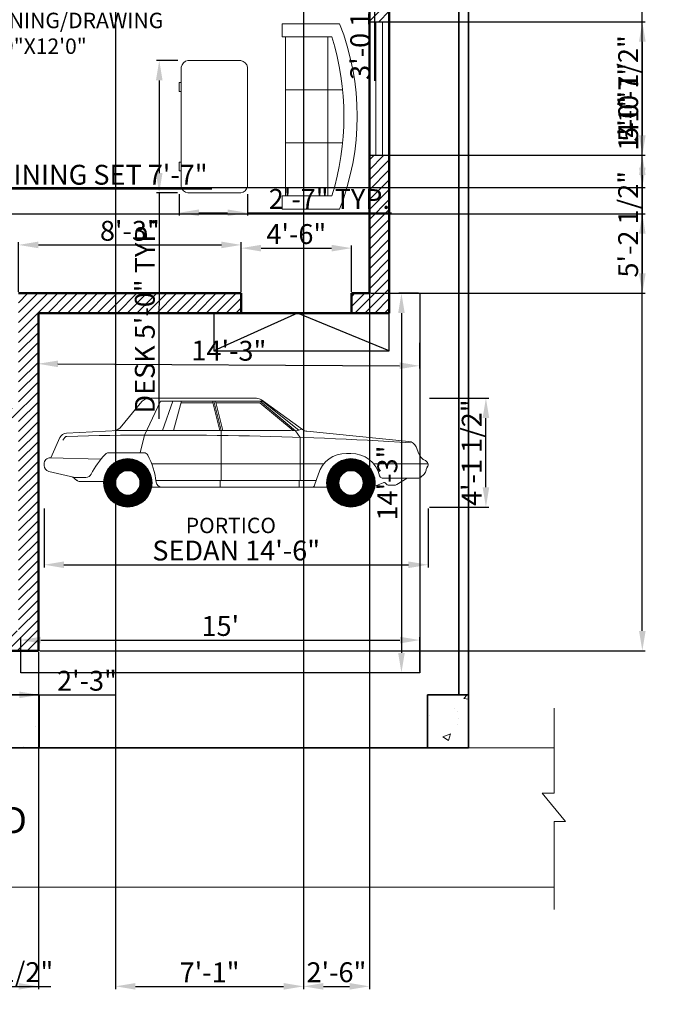
# Model space of a CAD drawing. Units: inches. Extents: x 53662 to 54269, y 37303 to 38048.
# Tile 4 of 6: x 53979 to 54269, y 37303 to 37749. Entities that reach past the tile are written whole.
import ezdxf

# ---------------------------------------------------------------- set-up
doc = ezdxf.new("R2010")
doc.units = ezdxf.units.IN
for name, color, linetype, lineweight in [('A-ANNO-DIMS', 2, 'Continuous', 18), ('A-ANNO-TEXT', 7, 'Continuous', 25), ('A-AREA-IDEN', 7, 'Continuous', 25), ('A-EQPM-VEHI', 8, 'Continuous', 13), ('A-FLOR', 7, 'Continuous', 25), ('A-FLOR-STRS', 7, 'Continuous', 25), ('A-FURN', 8, 'Continuous', 18), ('A-GLAZ', 4, 'Continuous', 18), ('A-WALL', 7, 'Continuous', 50), ('C-PROP', 7, 'Continuous', 35), ('C-ROAD', 8, 'Continuous', 18), ('C-SITE-PATT', 8, 'Continuous', 13)]:
    doc.layers.add(name, color=color, linetype=linetype, lineweight=lineweight)
doc.layers.add('A-WALL-PATT', color=244, linetype='Continuous', lineweight=13, true_color=0x991b1e)
doc.styles.get("Standard").update_dxf_attribs({"font": 'arial.ttf'})
doc.dimstyles.new('ISO-25', dxfattribs={"dimtxt": 9, "dimasz": 9, "dimexe": 1.25, "dimexo": 0.625, "dimtad": 1, "dimdec": 1, "dimrnd": 9, "dimlunit": 3, "dimtxsty": 'Standard', "dimcen": 2.5, "dimadec": 0, "dimazin": 0, "dimtfac": 1, "dimtdec": 1, "dimtmove": 0, "dimatfit": 3, "dimfxl": 1, "dimarcsym": 0})

# ---------------------------------------------------------------- blocks, each defined once
blk = doc.blocks.new('Car - sedan  side')
for p, q in [((-77.81, 49.34), (-126.58, 49.34)), ((-139.53, 35.99), (-129.64, 47.91)), ((-128.57, 32.64), (-121.22, 48.02)), ((-74.7, 48.02), (-121.22, 48.02)), ((-120.32, 34.67), (-115.67, 48.02)), ((-115.4, 34.67), (-111.74, 48.02)), ((-97.55, 47.3), (-111.94, 47.3)), ((-94.41, 34.67), (-97.73, 48.02)), ((-93.72, 34.67), (-97.04, 48.02)), ((-93.03, 34.67), (-96.34, 48.02)), ((-76.26, 47.3), (-96.16, 47.3)), ((-61.08, 34.66), (-76.26, 47.3)), ((-60.02, 34.65), (-76.07, 48.02)), ((-56.87, 35.13), (-75.48, 48.59)), ((-58.54, 34.93), (-74.99, 48.02)), ((-170.93, 22.32), (-166.81, 31.56)), ((-164.57, 31.6), (-165.48, 30.35)), ((-140.23, 34.67), (-163.88, 33.56)), ((-62.28, 34.67), (-140.23, 34.67)), ((-130.39, 24.63), (-128.57, 32.64)), ((-93.72, 19.62), (-93.72, 34.67)), ((-62.28, 34.67), (-60.02, 34.65)), ((-60.02, 34.65), (-58.54, 34.93)), ((-57.97, 31.61), (-60.02, 34.65)), ((-57.21, 35.38), (-58.54, 34.93)), ((-57.97, 19.62), (-57.97, 31.61)), ((-54.93, 34.4), (-8.75, 29.8)), ((-4.21, 24.18), (-5.42, 27.27)), ((-148.26, 21.7), (-171.11, 22.33)), ((-128.78, 24.63), (-144.79, 24.63)), ((-36.97, 24.38), (-34.94, 24.38)), ((-174, 19.51), (-174, 18.91)), ((-47.2, 19.62), (-125.23, 19.62)), ((-93.72, 12.14), (-93.72, 19.62)), ((-57.97, 12.14), (-57.97, 19.62)), ((0, 19.62), (-24.7, 19.62)), ((-160.12, 13.48), (-171.81, 16.16)), ((-159.22, 12.14), (-161.08, 13.7)), ((-155.01, 13.48), (-160.12, 13.48)), ((-51.4, 9.89), (-49.69, 15.14)), ((-3.22, 13.59), (-1.77, 14.97)), ((-147.03, 11.6), (-157.73, 11.6)), ((-120.62, 9.03), (-125.23, 9.03)), ((-50.67, 12.14), (-123.32, 12.14)), ((-45.76, 9.03), (-120.62, 9.03)), ((-94.21, 9.03), (-94.21, 12.14)), ((-58.39, 9.03), (-58.39, 12.14)), ((-20.36, 11.06), (-24.06, 9.44)), ((-4.23, 13.19), (-20.72, 13.19)), ((-18.83, 10.42), (-19.11, 10.76)), ((-14.68, 10.03), (-18.01, 10.03)), ((-9.5, 13.19), (-14.1, 10.2))]:
    blk.add_line(p, q)
at = {"const_width": 5.49}
for points in [[(-127.8, 11, -1), (-144.3, 11, -1)], [(-26.69, 11, -1), (-43.19, 11, -1)]]:
    blk.add_lwpolyline(points, format="xyb", close=True, dxfattribs=at)
for centre, radius in [((-136.05, 11), 11), ((-34.94, 11), 11), ((-136.05, 11), 5.51), ((-34.94, 11), 5.51)]:
    blk.add_circle(centre, radius)
for centre, radius, start, end in [((-126.58, 45.38), 3.97, 90, 140.3029), ((-77.81, 45.38), 3.97, 54.135, 90), ((-142.58, 38.53), 3.97, 272.6827, 320.3029), ((-163.72, 30.18), 3.38, 92.6827, 155.9736), ((-163.62, 30.91), 1.17, 91.491, 143.9553), ((-118.51, -1702.12), 1734.79, 86.34698, 91.49105), ((-54.54, 38.35), 3.97, 234.135, 264.3123), ((-9.15, 25.82), 4, 21.3107, 84.3123), ((-171.18, 19.51), 2.82, 88.4193, 180), ((-118.09, -2.78), 38.85, 136.3964, 152.9097), ((-144.79, 22.64), 1.98, 90, 136.3964), ((-128.78, 22.64), 1.98, 28.1371, 90), ((-157.14, 7.48), 34.14, 6.5135, 28.1371), ((-36.97, 11), 13.38, 90, 161.9732), ((-34.94, 11), 13.38, 13.5864, 90), ((0.9, 26.18), 5.49, 201.3107, 247.7048), ((-171.18, 18.91), 2.82, 180, 257.0905), ((-1.92, 19.3), 1.94, 325.3744, 67.7048), ((2.46, 16.28), 3.37, 145.3744, 172.3839), ((-155.01, 16.1), 2.62, 270, 332.9097), ((-20.72, 14.43), 1.24, 193.5864, 270), ((-4.23, 14.65), 1.46, 270, 313.7173), ((-3.82, 17.12), 2.96, 313.7173, 352.3839), ((-157.73, 13.93), 2.32, 230.1291, 270), ((-120.62, 11.65), 2.62, 186.5135, 270), ((-52.58, 10.27), 1.24, 270, 341.9732), ((-19.93, 10.09), 1.06, 39.301, 113.7159), ((-18.01, 11.09), 1.06, 219.301, 270), ((-14.68, 11.09), 1.06, 270, 303.047)]:
    blk.add_arc(centre, radius, start, end)
blk = doc.blocks.new('Sofa - Roundback 7 ft.')
for p, q in [((-12.00002, -32.4421), (-12.00003, -6.5971)), ((11.99997, -32.4421), (11.99998, -6.5971)), ((-36.000027, -34), (-36.000027, -11.4696)), ((-35.999844, -13.3819), (35.9998, -13.3819)), ((35.99998, -34), (35.99998, -11.4696)), ((-36.000027, -32.4421), (35.99998, -32.4421))]:
    blk.add_line(p, q)
for points in [[(-36.000027, -34), (-42.000027, -34), (-42.000027, -8)], [(41.99998, -8), (41.99998, -34), (35.99998, -34)]]:
    blk.add_lwpolyline(points)
for centre, radius, start, end in [((0, -114.25), 114.25, 68.43141, 111.5686), ((-0.00001, -127.1968), 121.1968, 72.72033, 107.2797)]:
    blk.add_arc(centre, radius, start, end)
blk = doc.blocks.new('Desk - 30 x 60 in.')
for p, q in [((-26.999995, 0), (26.999995, 0)), ((-29.999995, -27), (-29.999995, -3)), ((29.999995, -3), (29.999995, -27)), ((26.999995, -30), (-26.999995, -30)), ((-20.000005, -30), (-20.000005, -31)), ((-20.000005, -31), (-16.000005, -31)), ((-16.000005, -31), (-16.000005, -30)), ((15.999995, -31), (15.999995, -30)), ((19.999995, -31), (15.999995, -31)), ((19.999995, -30), (19.999995, -31))]:
    blk.add_line(p, q)
for centre, start, end in [((-26.499995, -3.5), 98.1301, 171.8699), ((26.499995, -3.5), 8.130102, 81.8699), ((-26.499995, -26.5), 188.1301, 261.8699), ((26.499995, -26.5), 278.1301, 351.8699)]:
    blk.add_arc(centre, 3.535534, start, end)
blk = doc.blocks.new('*D19')
at = {"layer": 'A-ANNO-DIMS', "color": 0, "lineweight": -2, "transparency": 16777216}
for p, q in [((53964.39, 37443.48), (53964.39, 37444.1)), ((53973.39, 37442.85), (53978.47, 37442.85)), ((53987.47, 37442.85), (54021.8, 37442.85)), ((53987.47, 37442.23), (53987.47, 37441.6))]:
    blk.add_line(p, q, dxfattribs=at)
at = {"layer": 'A-ANNO-DIMS', "color": 0, "transparency": 16777216}
for points in [[(53973.39, 37444.35), (53973.39, 37441.35), (53964.39, 37442.85)], [(53978.47, 37444.35), (53978.47, 37441.35), (53987.47, 37442.85)]]:
    blk.add_solid(points, dxfattribs=at)
at = {"layer": 'Defpoints', "color": 0, "transparency": 16777216}
for p in [(53964.39, 37442.85), (53987.47, 37442.85), (53987.47, 37442.85)]:
    blk.add_point(p, dxfattribs=at)
at = {"layer": 'A-ANNO-DIMS', "color": 0, "transparency": 16777216, "insert": (54009.13, 37448.08), "char_height": 9, "attachment_point": 5}
blk.add_mtext('2\'-3"', dxfattribs=at)
blk = doc.blocks.new('*D20')
at = {"layer": 'A-ANNO-DIMS', "color": 0, "lineweight": -2, "transparency": 16777216}
for p, q in [((53979.17, 37453.49), (53979.17, 37468.93)), ((53988.17, 37467.68), (54150.95, 37467.68)), ((54159.95, 37453.49), (54159.95, 37468.93))]:
    blk.add_line(p, q, dxfattribs=at)
at = {"layer": 'A-ANNO-DIMS', "color": 0, "transparency": 16777216}
for points in [[(53988.17, 37469.18), (53988.17, 37466.18), (53979.17, 37467.68)], [(54150.95, 37469.18), (54150.95, 37466.18), (54159.95, 37467.68)]]:
    blk.add_solid(points, dxfattribs=at)
at = {"layer": 'Defpoints', "color": 0, "transparency": 16777216}
for p in [(54159.95, 37467.68), (53979.17, 37452.86), (54159.95, 37452.86)]:
    blk.add_point(p, dxfattribs=at)
at = {"layer": 'A-ANNO-DIMS', "color": 0, "transparency": 16777216, "insert": (54069.56, 37472.9), "char_height": 9, "attachment_point": 5}
blk.add_mtext("15'", dxfattribs=at)
blk = doc.blocks.new('*D21')
at = {"layer": 'A-ANNO-DIMS', "color": 0, "lineweight": -2, "transparency": 16777216}
for p, q in [((54159.33, 37624.86), (54150.4, 37624.86)), ((54151.65, 37615.86), (54151.65, 37461.86)), ((54159.33, 37452.86), (54150.4, 37452.86))]:
    blk.add_line(p, q, dxfattribs=at)
at = {"layer": 'A-ANNO-DIMS', "color": 0, "transparency": 16777216}
for points in [[(54150.15, 37615.86), (54153.15, 37615.86), (54151.65, 37624.86)], [(54150.15, 37461.86), (54153.15, 37461.86), (54151.65, 37452.86)]]:
    blk.add_solid(points, dxfattribs=at)
at = {"layer": 'Defpoints', "color": 0, "transparency": 16777216}
for p in [(54159.95, 37624.86), (54151.65, 37452.86), (54159.95, 37452.86)]:
    blk.add_point(p, dxfattribs=at)
at = {"layer": 'A-ANNO-DIMS', "color": 0, "transparency": 16777216, "insert": (54146.43, 37538.86), "char_height": 9, "attachment_point": 5, "rotation": 90}
blk.add_mtext('14\'-3"', dxfattribs=at)
blk = doc.blocks.new('*D23')
at = {"layer": 'A-ANNO-DIMS', "color": 0, "lineweight": -2, "transparency": 16777216}
for p, q in [((53978.11, 37625.49), (53978.11, 37648.03)), ((53987.11, 37646.78), (54070.03, 37646.78)), ((54079.03, 37625.49), (54079.03, 37648.03))]:
    blk.add_line(p, q, dxfattribs=at)
at = {"layer": 'A-ANNO-DIMS', "color": 0, "transparency": 16777216}
for points in [[(53987.11, 37648.28), (53987.11, 37645.28), (53978.11, 37646.78)], [(54070.03, 37648.28), (54070.03, 37645.28), (54079.03, 37646.78)]]:
    blk.add_solid(points, dxfattribs=at)
at = {"layer": 'Defpoints', "color": 0, "transparency": 16777216}
for p in [(54079.03, 37646.78), (53978.11, 37624.86), (54079.03, 37624.86)]:
    blk.add_point(p, dxfattribs=at)
at = {"layer": 'A-ANNO-DIMS', "color": 0, "transparency": 16777216, "insert": (54028.57, 37652), "char_height": 9, "attachment_point": 5}
blk.add_mtext('8\'-3"', dxfattribs=at)
blk = doc.blocks.new('*D24')
at = {"layer": 'A-ANNO-DIMS', "color": 0, "lineweight": -2, "transparency": 16777216}
for p, q in [((54079.03, 37625.49), (54079.03, 37646.56)), ((54128.99, 37625.49), (54128.99, 37646.56)), ((54088.03, 37645.31), (54119.99, 37645.31))]:
    blk.add_line(p, q, dxfattribs=at)
at = {"layer": 'A-ANNO-DIMS', "color": 0, "transparency": 16777216}
for points in [[(54088.03, 37646.81), (54088.03, 37643.81), (54079.03, 37645.31)], [(54119.99, 37646.81), (54119.99, 37643.81), (54128.99, 37645.31)]]:
    blk.add_solid(points, dxfattribs=at)
at = {"layer": 'Defpoints', "color": 0, "transparency": 16777216}
for p in [(54128.99, 37645.31), (54079.03, 37624.86), (54128.99, 37624.86)]:
    blk.add_point(p, dxfattribs=at)
at = {"layer": 'A-ANNO-DIMS', "color": 0, "transparency": 16777216, "insert": (54104.01, 37650.53), "char_height": 9, "attachment_point": 5}
blk.add_mtext('4\'-6"', dxfattribs=at)
blk = doc.blocks.new('*D25')
at = {"layer": 'A-ANNO-DIMS', "color": 0, "lineweight": -2, "transparency": 16777216}
for p, q in [((53987.11, 37615.24), (53986.99, 37591.66)), ((54159.95, 37614.31), (54159.82, 37590.73)), ((53995.99, 37592.86), (54150.83, 37592.03))]:
    blk.add_line(p, q, dxfattribs=at)
at = {"layer": 'A-ANNO-DIMS', "color": 0, "transparency": 16777216}
for points in [[(53996, 37594.36), (53995.98, 37591.36), (53986.99, 37592.91)], [(54150.84, 37593.53), (54150.82, 37590.53), (54159.83, 37591.98)]]:
    blk.add_solid(points, dxfattribs=at)
at = {"layer": 'Defpoints', "color": 0, "transparency": 16777216}
for p in [(53987.11, 37615.86), (54159.95, 37614.93), (54159.83, 37591.98)]:
    blk.add_point(p, dxfattribs=at)
at = {"layer": 'A-ANNO-DIMS', "color": 0, "transparency": 16777216, "insert": (54073.44, 37597.67), "char_height": 9, "attachment_point": 5, "rotation": 359.6927}
blk.add_mtext('14\'-3"', dxfattribs=at)
blk = doc.blocks.new('*D31')
at = {"layer": 'A-ANNO-DIMS', "color": 0, "lineweight": -2, "transparency": 16777216}
for p, q in [((54127.43, 37843.84), (54140.66, 37843.84)), ((54139.41, 37834.84), (54139.41, 37816.17)), ((54127.43, 37807.17), (54140.66, 37807.17)), ((54139.41, 37807.17), (54139.41, 37721.1))]:
    blk.add_line(p, q, dxfattribs=at)
at = {"layer": 'A-ANNO-DIMS', "color": 0, "transparency": 16777216}
for points in [[(54137.91, 37834.84), (54140.91, 37834.84), (54139.41, 37843.84)], [(54137.91, 37816.17), (54140.91, 37816.17), (54139.41, 37807.17)]]:
    blk.add_solid(points, dxfattribs=at)
at = {"layer": 'Defpoints', "color": 0, "transparency": 16777216}
for p in [(54126.81, 37843.84), (54126.81, 37807.17), (54139.41, 37807.17)]:
    blk.add_point(p, dxfattribs=at)
at = {"layer": 'A-ANNO-DIMS', "color": 0, "transparency": 16777216, "insert": (54134.13, 37759.63), "char_height": 9, "attachment_point": 5, "rotation": 90}
blk.add_mtext('3\'-0 1/2" TYP.', dxfattribs=at)
blk = doc.blocks.new('*D32')
at = {"layer": 'A-ANNO-DIMS', "color": 0, "lineweight": -2, "transparency": 16777216}
for p, q in [((54050.27, 37730.35), (54040.65, 37730.36)), ((54041.89, 37721.36), (54041.86, 37679.36)), ((54050.23, 37670.35), (54040.6, 37670.36)), ((54041.85, 37670.36), (54041.77, 37567.96))]:
    blk.add_line(p, q, dxfattribs=at)
at = {"layer": 'A-ANNO-DIMS', "color": 0, "transparency": 16777216}
for points in [[(54040.39, 37721.36), (54043.39, 37721.35), (54041.9, 37730.36)], [(54040.36, 37679.36), (54043.36, 37679.35), (54041.85, 37670.36)]]:
    blk.add_solid(points, dxfattribs=at)
at = {"layer": 'Defpoints', "color": 0, "transparency": 16777216}
for p in [(54050.9, 37730.35), (54041.85, 37670.36), (54050.85, 37670.35)]:
    blk.add_point(p, dxfattribs=at)
at = {"layer": 'A-ANNO-DIMS', "color": 0, "transparency": 16777216, "insert": (54036.53, 37614.66), "char_height": 9, "attachment_point": 5, "rotation": 89.9534}
blk.add_mtext('DESK 5\'-0" TYP.', dxfattribs=at)
blk = doc.blocks.new('*D33')
at = {"layer": 'A-ANNO-DIMS', "color": 0, "lineweight": -2, "transparency": 16777216}
for p, q in [((54050.85, 37669.72), (54050.84, 37660.1)), ((54081.85, 37669.7), (54081.84, 37660.07)), ((54059.84, 37661.34), (54072.84, 37661.33)), ((54081.84, 37661.32), (54147.11, 37661.27))]:
    blk.add_line(p, q, dxfattribs=at)
at = {"layer": 'A-ANNO-DIMS', "color": 0, "transparency": 16777216}
for points in [[(54059.84, 37662.84), (54059.84, 37659.84), (54050.84, 37661.35)], [(54072.84, 37662.83), (54072.84, 37659.83), (54081.84, 37661.32)]]:
    blk.add_solid(points, dxfattribs=at)
at = {"layer": 'Defpoints', "color": 0, "transparency": 16777216}
for p in [(54050.85, 37670.35), (54081.85, 37670.32), (54081.84, 37661.32)]:
    blk.add_point(p, dxfattribs=at)
at = {"layer": 'A-ANNO-DIMS', "color": 0, "transparency": 16777216, "insert": (54118.98, 37666.44), "char_height": 9, "attachment_point": 5, "rotation": 359.9534}
blk.add_mtext('2\'-7" TYP.', dxfattribs=at)
blk = doc.blocks.new('*D34')
at = {"layer": 'A-ANNO-DIMS', "color": 0, "lineweight": -2, "transparency": 16777216}
for p, q in [((53865.53, 37685.16), (53865.53, 37670.88)), ((53956.53, 37685.16), (53956.53, 37670.88)), ((53874.53, 37672.13), (53947.53, 37672.13)), ((53956.53, 37672.13), (54065.7, 37672.13))]:
    blk.add_line(p, q, dxfattribs=at)
at = {"layer": 'A-ANNO-DIMS', "color": 0, "transparency": 16777216}
for points in [[(53874.53, 37673.63), (53874.53, 37670.63), (53865.53, 37672.13)], [(53947.53, 37673.63), (53947.53, 37670.63), (53956.53, 37672.13)]]:
    blk.add_solid(points, dxfattribs=at)
at = {"layer": 'Defpoints', "color": 0, "transparency": 16777216}
for p in [(53865.53, 37685.78), (53956.53, 37685.78), (53956.53, 37672.13)]:
    blk.add_point(p, dxfattribs=at)
at = {"layer": 'A-ANNO-DIMS', "color": 0, "transparency": 16777216, "insert": (54015.61, 37677.41), "char_height": 9, "attachment_point": 5}
blk.add_mtext('DINING SET 7\'-7"', dxfattribs=at)
blk = doc.blocks.new('*D48')
at = {"layer": 'A-ANNO-DIMS', "color": 0, "lineweight": -2, "transparency": 16777216}
for p, q in [((53989.7, 37527.31), (53989.7, 37500.56)), ((54163.81, 37527.31), (54163.81, 37500.56)), ((53998.7, 37501.81), (54154.81, 37501.81))]:
    blk.add_line(p, q, dxfattribs=at)
at = {"layer": 'A-ANNO-DIMS', "color": 0, "transparency": 16777216}
for points in [[(53998.7, 37503.31), (53998.7, 37500.31), (53989.7, 37501.81)], [(54154.81, 37503.31), (54154.81, 37500.31), (54163.81, 37501.81)]]:
    blk.add_solid(points, dxfattribs=at)
at = {"layer": 'Defpoints', "color": 0, "transparency": 16777216}
for p in [(53989.7, 37527.93), (54163.81, 37527.93), (54163.81, 37501.81)]:
    blk.add_point(p, dxfattribs=at)
at = {"layer": 'A-ANNO-DIMS', "color": 0, "transparency": 16777216, "insert": (54076.76, 37507.09), "char_height": 9, "attachment_point": 5}
blk.add_mtext('SEDAN 14\'-6"', dxfattribs=at)
blk = doc.blocks.new('*D49')
at = {"layer": 'A-ANNO-DIMS', "color": 0, "lineweight": -2, "transparency": 16777216}
for p, q in [((54164.44, 37577.28), (54191.18, 37577.28)), ((54189.93, 37536.93), (54189.93, 37568.28)), ((54164.44, 37527.93), (54191.18, 37527.93))]:
    blk.add_line(p, q, dxfattribs=at)
at = {"layer": 'A-ANNO-DIMS', "color": 0, "transparency": 16777216}
for points in [[(54188.43, 37568.28), (54191.43, 37568.28), (54189.93, 37577.28)], [(54188.43, 37536.93), (54191.43, 37536.93), (54189.93, 37527.93)]]:
    blk.add_solid(points, dxfattribs=at)
at = {"layer": 'Defpoints', "color": 0, "transparency": 16777216}
for p in [(54163.81, 37577.28), (54189.93, 37577.28), (54163.81, 37527.93)]:
    blk.add_point(p, dxfattribs=at)
at = {"layer": 'A-ANNO-DIMS', "color": 0, "transparency": 16777216, "insert": (54184.65, 37552.6), "char_height": 9, "attachment_point": 5, "rotation": 90}
blk.add_mtext('4\'-1 1/2"', dxfattribs=at)
blk = doc.blocks.new('*D51')
at = {"layer": 'A-ANNO-DIMS', "color": 0, "lineweight": -2, "transparency": 16777216}
for p, q in [((54146.74, 37961.86), (54262.07, 37961.86)), ((54260.82, 37471.86), (54260.82, 37952.86)), ((53987.74, 37462.86), (54262.07, 37462.86))]:
    blk.add_line(p, q, dxfattribs=at)
at = {"layer": 'A-ANNO-DIMS', "color": 0, "transparency": 16777216}
for points in [[(54259.32, 37952.86), (54262.32, 37952.86), (54260.82, 37961.86)], [(54259.32, 37471.86), (54262.32, 37471.86), (54260.82, 37462.86)]]:
    blk.add_solid(points, dxfattribs=at)
at = {"layer": 'Defpoints', "color": 0, "transparency": 16777216}
for p in [(54146.11, 37961.86), (54260.82, 37961.86), (53987.11, 37462.86)]:
    blk.add_point(p, dxfattribs=at)
at = {"layer": 'A-ANNO-DIMS', "color": 0, "transparency": 16777216, "insert": (54255.68, 37712.36), "char_height": 9, "attachment_point": 5, "rotation": 90}
blk.add_mtext('41\'-7"', dxfattribs=at)
blk = doc.blocks.new('*D53')
at = {"layer": 'A-ANNO-DIMS', "color": 0, "lineweight": -2, "transparency": 16777216}
for p, q in [((54260.82, 37681.86), (54260.82, 37715.19)), ((53828.74, 37672.86), (54262.07, 37672.86)), ((54260.82, 37660.86), (54260.82, 37672.86)), ((53828.74, 37660.86), (54262.07, 37660.86)), ((54260.82, 37651.86), (54260.82, 37642.86))]:
    blk.add_line(p, q, dxfattribs=at)
at = {"layer": 'A-ANNO-DIMS', "color": 0, "transparency": 16777216}
for points in [[(54259.32, 37681.86), (54262.32, 37681.86), (54260.82, 37672.86)], [(54259.32, 37651.86), (54262.32, 37651.86), (54260.82, 37660.86)]]:
    blk.add_solid(points, dxfattribs=at)
at = {"layer": 'Defpoints', "color": 0, "transparency": 16777216}
for p in [(53828.11, 37672.86), (54260.82, 37672.86), (53828.11, 37660.86)]:
    blk.add_point(p, dxfattribs=at)
at = {"layer": 'A-ANNO-DIMS', "color": 0, "transparency": 16777216, "insert": (54255.6, 37703.02), "char_height": 9, "attachment_point": 5, "rotation": 90}
blk.add_mtext('1\'-0"', dxfattribs=at)
blk = doc.blocks.new('*D58')
at = {"layer": 'A-ANNO-DIMS', "color": 0, "lineweight": -2, "transparency": 16777216}
for p, q in [((54022.12, 37952.24), (54022.12, 37309.49)), ((54107.27, 37952.24), (54107.27, 37309.49)), ((54031.12, 37310.74), (54098.27, 37310.74))]:
    blk.add_line(p, q, dxfattribs=at)
at = {"layer": 'A-ANNO-DIMS', "color": 0, "transparency": 16777216}
for points in [[(54031.12, 37312.24), (54031.12, 37309.24), (54022.12, 37310.74)], [(54098.27, 37312.24), (54098.27, 37309.24), (54107.27, 37310.74)]]:
    blk.add_solid(points, dxfattribs=at)
at = {"layer": 'Defpoints', "color": 0, "transparency": 16777216}
for p in [(54022.12, 37952.86), (54107.27, 37952.86), (54107.27, 37310.74)]:
    blk.add_point(p, dxfattribs=at)
at = {"layer": 'A-ANNO-DIMS', "color": 0, "transparency": 16777216, "insert": (54064.7, 37315.88), "char_height": 9, "attachment_point": 5}
blk.add_mtext('7\'-1"', dxfattribs=at)
blk = doc.blocks.new('*D59')
at = {"layer": 'A-ANNO-DIMS', "color": 0, "lineweight": -2, "transparency": 16777216}
for p, q in [((54107.27, 37952.24), (54107.27, 37309.49)), ((54137.11, 37952.24), (54137.11, 37309.49)), ((54116.27, 37310.74), (54128.11, 37310.74))]:
    blk.add_line(p, q, dxfattribs=at)
at = {"layer": 'A-ANNO-DIMS', "color": 0, "transparency": 16777216}
for points in [[(54116.27, 37312.24), (54116.27, 37309.24), (54107.27, 37310.74)], [(54128.11, 37312.24), (54128.11, 37309.24), (54137.11, 37310.74)]]:
    blk.add_solid(points, dxfattribs=at)
at = {"layer": 'Defpoints', "color": 0, "transparency": 16777216}
for p in [(54107.27, 37952.86), (54137.11, 37952.86), (54137.11, 37310.74)]:
    blk.add_point(p, dxfattribs=at)
at = {"layer": 'A-ANNO-DIMS', "color": 0, "transparency": 16777216, "insert": (54122.19, 37315.96), "char_height": 9, "attachment_point": 5}
blk.add_mtext('2\'-6"', dxfattribs=at)
blk = doc.blocks.new('*D60')
at = {"layer": 'A-ANNO-DIMS', "color": 0, "lineweight": -2, "transparency": 16777216}
for p, q in [((53924.11, 37790.24), (53924.11, 37309.49)), ((53928.61, 37790.24), (53928.61, 37309.49)), ((53915.11, 37310.74), (53906.11, 37310.74)), ((53924.11, 37310.74), (53928.61, 37310.74)), ((53937.61, 37310.74), (53992.76, 37310.74))]:
    blk.add_line(p, q, dxfattribs=at)
at = {"layer": 'A-ANNO-DIMS', "color": 0, "transparency": 16777216}
for points in [[(53915.11, 37312.24), (53915.11, 37309.24), (53924.11, 37310.74)], [(53937.61, 37312.24), (53937.61, 37309.24), (53928.61, 37310.74)]]:
    blk.add_solid(points, dxfattribs=at)
at = {"layer": 'Defpoints', "color": 0, "transparency": 16777216}
for p in [(53924.11, 37790.86), (53928.61, 37790.86), (53928.61, 37310.74)]:
    blk.add_point(p, dxfattribs=at)
at = {"layer": 'A-ANNO-DIMS', "color": 0, "transparency": 16777216, "insert": (53969.69, 37316.02), "char_height": 9, "attachment_point": 5}
blk.add_mtext('0\'-4 1/2"', dxfattribs=at)
blk = doc.blocks.new('*D68')
at = {"layer": 'A-ANNO-DIMS', "color": 0, "lineweight": -2, "transparency": 16777216}
for p, q in [((54137.74, 37747.89), (54262.07, 37747.89)), ((54260.82, 37738.89), (54260.82, 37696.42)), ((54137.74, 37687.42), (54262.07, 37687.42))]:
    blk.add_line(p, q, dxfattribs=at)
at = {"layer": 'A-ANNO-DIMS', "color": 0, "transparency": 16777216}
for points in [[(54259.32, 37738.89), (54262.32, 37738.89), (54260.82, 37747.89)], [(54259.32, 37696.42), (54262.32, 37696.42), (54260.82, 37687.42)]]:
    blk.add_solid(points, dxfattribs=at)
at = {"layer": 'Defpoints', "color": 0, "transparency": 16777216}
for p in [(54137.11, 37747.89), (54137.11, 37687.42), (54260.82, 37687.42)]:
    blk.add_point(p, dxfattribs=at)
at = {"layer": 'A-ANNO-DIMS', "color": 0, "transparency": 16777216, "insert": (54255.55, 37717.66), "char_height": 9, "attachment_point": 5, "rotation": 90}
blk.add_mtext('5\'-0 1/2"', dxfattribs=at)
blk = doc.blocks.new('*D69')
at = {"layer": 'A-ANNO-DIMS', "color": 0, "lineweight": -2, "transparency": 16777216}
for p, q in [((54137.74, 37687.42), (54262.07, 37687.42)), ((54260.82, 37678.42), (54260.82, 37633.86)), ((54137.74, 37624.86), (54262.07, 37624.86))]:
    blk.add_line(p, q, dxfattribs=at)
at = {"layer": 'A-ANNO-DIMS', "color": 0, "transparency": 16777216}
for points in [[(54259.32, 37678.42), (54262.32, 37678.42), (54260.82, 37687.42)], [(54259.32, 37633.86), (54262.32, 37633.86), (54260.82, 37624.86)]]:
    blk.add_solid(points, dxfattribs=at)
at = {"layer": 'Defpoints', "color": 0, "transparency": 16777216}
for p in [(54137.11, 37687.42), (54137.11, 37624.86), (54260.82, 37624.86)]:
    blk.add_point(p, dxfattribs=at)
at = {"layer": 'A-ANNO-DIMS', "color": 0, "transparency": 16777216, "insert": (54255.55, 37656.14), "char_height": 9, "attachment_point": 5, "rotation": 90}
blk.add_mtext('5\'-2 1/2"', dxfattribs=at)
blk = doc.blocks.new('*D71')
at = {"layer": 'A-ANNO-DIMS', "color": 0, "lineweight": -2, "transparency": 16777216}
for p, q in [((53926.17, 37462.24), (53926.17, 37309.49)), ((53987.11, 37462.24), (53987.11, 37309.49)), ((53935.17, 37310.74), (53978.11, 37310.74))]:
    blk.add_line(p, q, dxfattribs=at)
at = {"layer": 'A-ANNO-DIMS', "color": 0, "transparency": 16777216}
for points in [[(53935.17, 37312.24), (53935.17, 37309.24), (53926.17, 37310.74)], [(53978.11, 37312.24), (53978.11, 37309.24), (53987.11, 37310.74)]]:
    blk.add_solid(points, dxfattribs=at)
at = {"layer": 'Defpoints', "color": 0, "transparency": 16777216}
for p in [(53926.17, 37462.86), (53987.11, 37462.86), (53987.11, 37310.74)]:
    blk.add_point(p, dxfattribs=at)
at = {"layer": 'A-ANNO-DIMS', "color": 0, "transparency": 16777216, "insert": (53956.64, 37315.96), "char_height": 9, "attachment_point": 5}
blk.add_mtext('5\'-1"', dxfattribs=at)

msp = doc.modelspace()

# ---------------------------------------------------------------- hatches: boundary and pattern name
at = {"layer": 'A-WALL-PATT'}
h = msp.add_hatch(dxfattribs=at)
h.set_pattern_fill('ANSI31', color=256)
h.paths.add_polyline_path([(53792.11, 37952.86), (53849.2, 37952.86), (53849.2, 37961.86), (53783.11, 37961.86), (53783.11, 37861.42), (53792.11, 37861.42)])
h.paths.add_polyline_path([(53940.97, 37961.86), (53893.52, 37961.86), (53893.52, 37952.86), (53924.11, 37952.86), (53924.11, 37921.83), (53926.36, 37921.83, -0.026334), (53928.61, 37921.99), (53928.61, 37930.37), (53928.61, 37952.86), (53940.97, 37952.86)])
h.paths.add_polyline_path([(53792.11, 37786.36), (53882.05, 37786.36), (53882.05, 37788.61, -0.017862), (53881.82, 37790.86), (53792.11, 37790.86), (53792.11, 37806.76), (53783.11, 37806.76), (53783.11, 37732.86), (53792.11, 37732.86)])
h.paths.add_polyline_path([(53792.11, 37672.86), (53783.11, 37672.86), (53783.11, 37615.86), (53804.11, 37615.86), (53804.11, 37599.43), (53813.11, 37599.43), (53813.11, 37620.36), (53922.61, 37620.36), (53922.61, 37624.86), (53792.11, 37624.86)])
h.paths.add_polyline_path([(53978.11, 37572.86), (53927.11, 37572.86), (53927.11, 37620.36), (53922.61, 37620.36), (53922.61, 37568.36), (53978.11, 37568.36)])
h.paths.add_polyline_path([(53927.11, 37624.86), (53922.61, 37624.86), (53922.61, 37620.36), (53927.11, 37620.36)])
h.paths.add_polyline_path([(53987.11, 37615.86), (54079.03, 37615.86), (54079.03, 37624.86), (53978.11, 37624.86), (53978.11, 37471.86), (53926.17, 37471.86), (53926.17, 37462.86), (53987.11, 37462.86)])
h.paths.add_polyline_path([(53813.11, 37561.58), (53804.11, 37561.58), (53804.11, 37471.86), (53783.11, 37471.86), (53783.11, 37462.86), (53873.85, 37462.86), (53873.85, 37471.86), (53813.11, 37471.86)])
h.paths.add_polyline_path([(54146.11, 37687.42), (54137.11, 37687.42), (54137.11, 37624.86), (54128.99, 37624.86), (54128.99, 37615.86), (54146.11, 37615.86)])
h.paths.add_polyline_path([(54146.11, 37813.18), (54137.11, 37813.18), (54137.11, 37747.89), (54146.11, 37747.89)])
h.paths.add_polyline_path([(54146.11, 37961.86), (54107.27, 37961.86), (54107.27, 37952.86), (54137.11, 37952.86), (54137.11, 37884.55), (54146.11, 37884.55)])
h.paths.add_polyline_path([(54022.12, 37961.86), (53964.61, 37961.86), (53964.61, 37952.86), (53982.61, 37952.86), (53982.61, 37822.8), (53987.11, 37822.8), (53987.11, 37952.86), (54022.12, 37952.86)])
h.paths.add_polyline_path([(53928.61, 37899.06), (53924.11, 37899.06), (53924.11, 37790.86), (53914.92, 37790.86), (53914.92, 37786.36), (53987.11, 37786.36), (53987.11, 37797.48), (53982.61, 37797.48), (53982.61, 37790.86), (53928.61, 37790.86), (53928.61, 37801.6, -0.072813), (53928.13, 37805.9, -0.05664), (53928.61, 37809.23)])
at = {"layer": 'C-SITE-PATT'}
h = msp.add_hatch(dxfattribs=at)
h.set_pattern_fill('AR-CONC', color=256, scale=0.2)
h.paths.add_polyline_path([(54182.11, 37442.85), (54163.41, 37442.85), (54163.41, 37418.86), (54182.11, 37418.86)])
h.paths.add_polyline_path([(53987.47, 37442.85), (53964.39, 37442.85), (53964.39, 37418.86), (53987.47, 37418.86)])

# ---------------------------------------------------------------- linework, layer by layer
at = {"layer": 'A-FLOR'}
for p, q in [((54146.11, 37624.86), (54159.95, 37624.86)), ((54159.95, 37624.86), (54159.95, 37452.86)), ((53979.17, 37452.86), (53979.17, 37462.86)), ((54159.95, 37452.86), (53979.17, 37452.86))]:
    msp.add_line(p, q, dxfattribs=at)
at = {"layer": 'A-FLOR-STRS'}
for p, q in [((54066.61, 37615.86), (54066.61, 37598.78)), ((54104.49, 37615.86), (54066.61, 37598.78)), ((54146.11, 37598.78), (54104.49, 37615.86)), ((54146.11, 37598.78), (54146.11, 37615.86)), ((54066.61, 37598.78), (54146.11, 37598.78))]:
    msp.add_line(p, q, dxfattribs=at)
at = {"layer": 'A-GLAZ'}
for p, q in [((54146.11, 37747.89), (54137.11, 37747.89)), ((54140.11, 37687.42), (54140.11, 37747.89)), ((54143.11, 37687.42), (54143.11, 37747.89)), ((54146.11, 37687.42), (54137.11, 37687.42))]:
    msp.add_line(p, q, dxfattribs=at)
at = {"layer": 'A-WALL'}
for p, q in [((54146.11, 37615.86), (54146.11, 37961.86)), ((54137.11, 37624.86), (54137.11, 37952.86)), ((54079.03, 37624.86), (53978.11, 37624.86)), ((54079.03, 37624.86), (54079.03, 37615.86)), ((54137.11, 37624.86), (54128.99, 37624.86)), ((54128.99, 37624.86), (54128.99, 37615.86)), ((54146.11, 37615.86), (53987.11, 37615.86)), ((53987.11, 37462.86), (53987.11, 37615.86)), ((53987.11, 37462.86), (53783.11, 37462.86))]:
    msp.add_line(p, q, dxfattribs=at)
at = {"layer": 'C-PROP'}
for p, q in [((54182.11, 37418.86), (54182.11, 37994.86)), ((54177.61, 37442.85), (54177.61, 37990.36)), ((53987.47, 37442.85), (53964.39, 37442.85)), ((53987.47, 37418.86), (53987.47, 37442.85)), ((54182.11, 37442.85), (54163.41, 37442.85)), ((54163.41, 37442.85), (54163.41, 37418.86)), ((53750.11, 37418.86), (54182.11, 37418.86))]:
    msp.add_line(p, q, dxfattribs=at)
at = {"layer": 'C-ROAD'}
for p, q in [((54220.88, 37436.83), (54220.88, 37398.28)), ((54182.11, 37418.86), (54220.88, 37418.86)), ((54220.88, 37398.28), (54215.48, 37398.28)), ((54215.48, 37398.28), (54225.97, 37385.45)), ((54225.97, 37385.45), (54220.88, 37385.45)), ((54220.88, 37385.45), (54220.88, 37345.59)), ((53718.77, 37355.76), (54220.88, 37355.76))]:
    msp.add_line(p, q, dxfattribs=at)

# ---------------------------------------------------------------- block references
at = {"layer": 'A-EQPM-VEHI'}
msp.add_blockref('Car - sedan  side', (54163.7, 37527.93), dxfattribs=at)
at = {"layer": 'A-FURN'}
for name, p, rotation in [('Sofa - Roundback 7 ft.', (54131.61, 37705.03), 270), ('Desk - 30 x 60 in.', (54081.87, 37700.32), 269.9533541638235)]:
    msp.add_blockref(name, p, dxfattribs=dict(at, rotation=rotation))

# ---------------------------------------------------------------- texts
at = {"layer": 'A-ANNO-TEXT', "insert": (53808.35, 37392.06), "char_height": 12, "attachment_point": 1}
msp.add_mtext_dynamic_manual_height_columns('30\'0" WIDE EAST ROAD', width=314.7476, gutter_width=12.5, heights=[0], dxfattribs=at)
at = {"layer": 'A-AREA-IDEN', "char_height": 7, "attachment_point": 1}
for s, width, insert in [('DINNING/DRAWING\\P21\'9"X12\'0"', 148.2626, (53957.4, 37752.01)), ('PORTICO', 60.1737, (54053.9, 37523.13))]:
    msp.add_mtext_dynamic_manual_height_columns(s, width=width, gutter_width=12.5, heights=[0], dxfattribs=dict(at, insert=insert))

# ---------------------------------------------------------------- dimensions: what is measured, and where the dimension line sits
at = {"layer": 'A-ANNO-DIMS'}
for base, p1, p2, override, picture, middle in [((54260.82, 37961.86), (53987.11, 37462.86), (54146.11, 37961.86), {"dimdec": 1, "dimlfac": 1, "dimrnd": 0, "dimzin": 1, "dimdsep": 46, "dimlunit": 4, "dimfrac": 2}, '*D51', (54255.68, 37712.36)), ((54260.82, 37687.42), (54137.11, 37747.89), (54137.11, 37687.42), {"dimdec": 1, "dimlfac": 1, "dimrnd": 0, "dimzin": 1, "dimdsep": 46, "dimlunit": 4, "dimfrac": 2}, '*D68', (54255.55, 37717.66)), ((54260.82, 37672.86), (53828.11, 37660.86), (53828.11, 37672.86), {"dimdec": 1, "dimlfac": 1, "dimrnd": 0, "dimzin": 1, "dimdsep": 46, "dimlunit": 4, "dimfrac": 2}, '*D53', (54255.6, 37703.02)), ((54260.82, 37624.86), (54137.11, 37687.42), (54137.11, 37624.86), {"dimdec": 1, "dimlfac": 1, "dimrnd": 0, "dimzin": 1, "dimdsep": 46, "dimlunit": 4, "dimfrac": 2}, '*D69', (54255.55, 37656.14)), ((54151.65, 37452.86), (54159.95, 37624.86), (54159.95, 37452.86), {"dimclrd": 0, "dimclre": 0, "dimclrt": 0}, '*D21', (54146.43, 37538.86)), ((54189.9309, 37577.2754), (54163.8138, 37527.9305), (54163.8138, 37577.2754), {"dimdec": 1, "dimlfac": 1, "dimrnd": 0, "dimzin": 1, "dimdsep": 46, "dimlunit": 4, "dimfrac": 2}, '*D49', (54184.6524, 37552.603))]:
    dim = msp.add_linear_dim(base=base, p1=p1, p2=p2, angle=90, dimstyle='ISO-25', override=override, dxfattribs=at)
    dim.commit()
    dim.dimension.update_dxf_attribs({"geometry": picture, "text_midpoint": middle})
for base, p1, p2, override, picture, middle in [((54107.2677, 37310.7389), (54022.1239, 37952.8602), (54107.2677, 37952.8602), {"dimdec": 1, "dimlfac": 1, "dimrnd": 0, "dimzin": 1, "dimdsep": 46, "dimlunit": 4, "dimfrac": 2}, '*D58', (54064.6958, 37315.8823)), ((54137.11, 37310.74), (54107.27, 37952.86), (54137.11, 37952.86), {"dimdec": 1, "dimlfac": 1, "dimrnd": 0, "dimzin": 1, "dimdsep": 46, "dimlunit": 4, "dimfrac": 2}, '*D59', (54122.19, 37315.96)), ((53928.61, 37310.74), (53924.11, 37790.86), (53928.61, 37790.86), {"dimdec": 1, "dimlfac": 1, "dimrnd": 0, "dimzin": 1, "dimdsep": 46, "dimlunit": 4, "dimfrac": 2}, '*D60', (53969.69, 37316.02)), ((54079.03, 37646.78), (53978.11, 37624.86), (54079.03, 37624.86), {"dimclrd": 0, "dimclre": 0, "dimclrt": 0}, '*D23', (54028.57, 37652)), ((54128.99, 37645.31), (54079.03, 37624.86), (54128.99, 37624.86), {"dimclrd": 0, "dimclre": 0, "dimclrt": 0}, '*D24', (54104.01, 37650.53)), ((54159.95, 37467.68), (53979.17, 37452.86), (54159.95, 37452.86), {"dimclrd": 0, "dimclre": 0, "dimclrt": 0}, '*D20', (54069.56, 37472.9)), ((53987.11, 37310.74), (53926.17, 37462.86), (53987.11, 37462.86), {"dimdec": 1, "dimlfac": 1, "dimrnd": 0, "dimzin": 1, "dimdsep": 46, "dimlunit": 4, "dimfrac": 2}, '*D71', (53956.64, 37315.96)), ((53987.47, 37442.85), (53964.39, 37442.85), (53987.47, 37442.85), {"dimclrd": 0, "dimclre": 0, "dimclrt": 0}, '*D19', (54009.13, 37448.08))]:
    dim = msp.add_linear_dim(base=base, p1=p1, p2=p2, dimstyle='ISO-25', override=override, dxfattribs=at)
    dim.commit()
    dim.dimension.update_dxf_attribs({"geometry": picture, "text_midpoint": middle})
for base, p1, p2, angle, text, picture, middle in [((54139.41, 37807.17), (54126.81, 37843.84), (54126.81, 37807.17), 270, '<> TYP.', '*D31', (54134.13, 37759.63)), ((54041.85, 37670.36), (54050.9, 37730.35), (54050.85, 37670.35), 269.9534, 'DESK <> TYP.', '*D32', (54036.53, 37614.66)), ((54081.84, 37661.32), (54050.85, 37670.35), (54081.85, 37670.32), 359.9534, '<> TYP.', '*D33', (54118.98, 37666.44))]:
    dim = msp.add_linear_dim(base=base, p1=p1, p2=p2, angle=angle, text=text, dimstyle='ISO-25', override={"dimdec": 1, "dimlfac": 1, "dimrnd": 0, "dimzin": 1, "dimdsep": 46, "dimlunit": 4, "dimfrac": 2}, dxfattribs=at)
    dim.commit()
    dim.dimension.update_dxf_attribs({"geometry": picture, "text_midpoint": middle})
for base, p1, p2, text, picture, middle in [((53956.53, 37672.13), (53865.53, 37685.78), (53956.53, 37685.78), 'DINING SET <>', '*D34', (54015.61, 37677.41)), ((54163.81, 37501.81), (53989.7, 37527.93), (54163.81, 37527.93), 'SEDAN <>', '*D48', (54076.76, 37507.09))]:
    dim = msp.add_linear_dim(base=base, p1=p1, p2=p2, text=text, dimstyle='ISO-25', override={"dimdec": 1, "dimlfac": 1, "dimrnd": 0, "dimzin": 1, "dimdsep": 46, "dimlunit": 4, "dimfrac": 2}, dxfattribs=at)
    dim.commit()
    dim.dimension.update_dxf_attribs({"geometry": picture, "text_midpoint": middle})
dim = msp.add_aligned_dim(p1=(53987.11, 37615.86), p2=(54159.95, 37614.93), distance=-22.95, dimstyle='ISO-25', override={"dimclrd": 0, "dimclre": 0, "dimclrt": 0}, dxfattribs=at)
dim.commit()
dim.dimension.update_dxf_attribs({"geometry": '*D25', "text_midpoint": (54073.44, 37597.67)})

doc.saveas('drawing.dxf')
